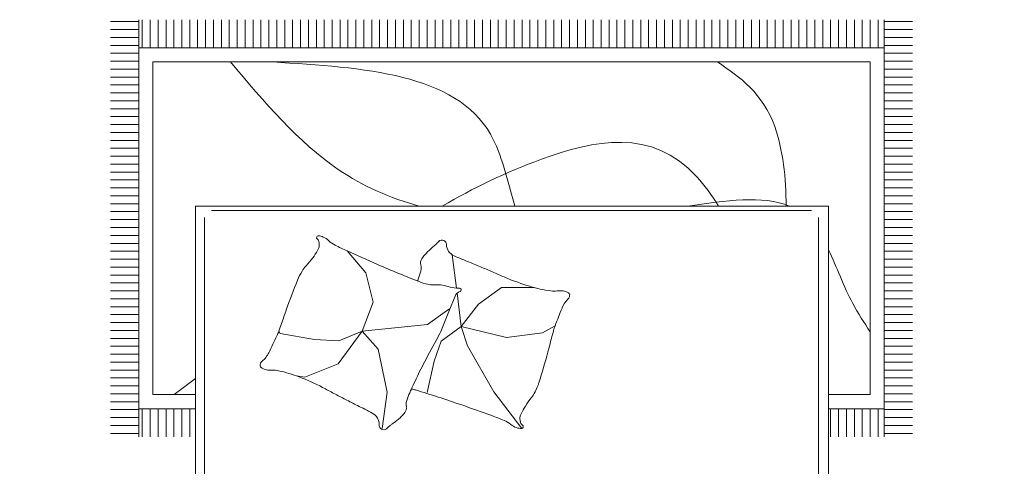
# Model space of a CAD drawing. Units: inches. Extents: x -7 to 1228, y -146 to 1091.
# Tile 46 of 88: x 81 to 168, y 616 to 655. Entities that reach past the tile are written whole.
import ezdxf

# ---------------------------------------------------------------- set-up
doc = ezdxf.new("R2010")
doc.units = ezdxf.units.IN
doc.layers.add('A-FURN', color=8, linetype='Continuous', lineweight=18)
doc.styles.add('DIM_FONT', font='SIMPLEX.shx', dxfattribs={"width": 0.8})

# ---------------------------------------------------------------- blocks, each defined once
blk = doc.blocks.new('A$C4F634EDD')
for p, q in [((0, 2.6295), (0, 2.2295)), ((0.5, 2.6295), (0, 2.6295)), ((0.5, 2.6295), (2.3, 2.6295)), ((0.5, 0.5295), (0.5, 2.6295)), ((0.5, 2.2295), (0.5, 2.6295)), ((2.3, 2.6295), (2.3, 0.5295)), ((2.3, 2.6295), (2.8, 2.6295)), ((2.3, 2.2295), (2.3, 2.6295)), ((2.8, 2.6295), (2.8, 2.2295)), ((0.5, 2.5771), (2.3, 2.5771)), ((2.392, 2.5115), (2.5692, 2.5765)), ((2.5692, 2.5765), (2.574, 2.5743)), ((0.2457, 2.5697), (0.2457, 2.4733)), ((2.4985, 2.5445), (2.5516, 2.564)), ((2.5062, 2.5454), (2.5487, 2.561)), ((2.5483, 2.5347), (2.5487, 2.561)), ((2.5487, 2.561), (2.5571, 2.56)), ((2.5615, 2.5536), (2.5514, 2.5318)), ((2.5516, 2.564), (2.5637, 2.5584)), ((2.5571, 2.56), (2.5615, 2.5536)), ((2.5615, 2.5536), (2.5791, 2.5058)), ((2.5637, 2.5584), (2.6418, 2.3458)), ((2.574, 2.5743), (2.6638, 2.3298)), ((2.4842, 2.5232), (2.47, 2.518)), ((2.4862, 2.5179), (2.4842, 2.5232)), ((2.4946, 2.5331), (2.4985, 2.5445)), ((2.5734, 2.3187), (2.4946, 2.5331)), ((2.5062, 2.5454), (2.5004, 2.5392)), ((2.5004, 2.5392), (2.5013, 2.5315)), ((2.5013, 2.5315), (2.5188, 2.4836)), ((2.5013, 2.5315), (2.5231, 2.5214)), ((2.5235, 2.5256), (2.5062, 2.5454)), ((2.5231, 2.5214), (2.5235, 2.5256)), ((2.5523, 2.4417), (2.5231, 2.5214)), ((2.5483, 2.5347), (2.5235, 2.5256)), ((2.5514, 2.5318), (2.5483, 2.5347)), ((2.5807, 2.4521), (2.5514, 2.5318)), ((2.3898, 2.5066), (2.392, 2.5115)), ((2.4795, 2.2621), (2.3898, 2.5066)), ((2.412, 2.5007), (2.4634, 2.5196)), ((2.4361, 2.4352), (2.412, 2.5007)), ((2.4634, 2.5196), (2.4875, 2.454)), ((2.47, 2.518), (2.472, 2.5127)), ((2.472, 2.5127), (2.4862, 2.5179)), ((2.4881, 2.5126), (2.4739, 2.5074)), ((2.4739, 2.5074), (2.4759, 2.502)), ((2.4759, 2.502), (2.4901, 2.5073)), ((2.492, 2.5019), (2.4778, 2.4967)), ((2.4778, 2.4967), (2.4798, 2.4914)), ((2.4798, 2.4914), (2.494, 2.4966)), ((2.4901, 2.5073), (2.4881, 2.5126)), ((2.494, 2.4966), (2.492, 2.5019)), ((2.5788, 2.4956), (2.5767, 2.4848)), ((2.5791, 2.5058), (2.5788, 2.4956)), ((2.4959, 2.4913), (2.4817, 2.4861)), ((2.4817, 2.4861), (2.4837, 2.4808)), ((2.4837, 2.4808), (2.4979, 2.486)), ((2.4998, 2.4807), (2.4856, 2.4755)), ((2.4856, 2.4755), (2.4876, 2.4702)), ((2.4876, 2.4702), (2.5018, 2.4754)), ((2.5037, 2.47), (2.4895, 2.4648)), ((2.4895, 2.4648), (2.4915, 2.4595)), ((2.4915, 2.4595), (2.5057, 2.4647)), ((2.4979, 2.486), (2.4959, 2.4913)), ((2.5018, 2.4754), (2.4998, 2.4807)), ((2.5057, 2.4647), (2.5037, 2.47)), ((2.5188, 2.4836), (2.5256, 2.4761)), ((2.5256, 2.4761), (2.5342, 2.4692)), ((2.5342, 2.4692), (2.5405, 2.4574)), ((2.5767, 2.4848), (2.5795, 2.4717)), ((2.5795, 2.4717), (2.586, 2.454)), ((2.4875, 2.454), (2.4361, 2.4352)), ((2.5405, 2.4574), (2.547, 2.4397)), ((2.5594, 2.4061), (2.547, 2.4397)), ((2.5523, 2.4417), (2.5875, 2.346)), ((2.5807, 2.4521), (2.6158, 2.3564)), ((2.5984, 2.4204), (2.586, 2.454)), ((0.0957, 2.4197), (0.192, 2.4197)), ((0.2994, 2.4197), (0.3957, 2.4197)), ((2.4457, 2.4146), (2.4563, 2.4185)), ((2.4496, 2.4039), (2.4457, 2.4146)), ((2.4563, 2.4185), (2.4602, 2.4078)), ((2.4634, 2.4211), (2.474, 2.425)), ((2.4673, 2.4104), (2.4634, 2.4211)), ((2.4779, 2.4143), (2.4673, 2.4104)), ((2.474, 2.425), (2.4779, 2.4143)), ((2.4811, 2.4276), (2.4917, 2.4315)), ((2.485, 2.4169), (2.4811, 2.4276)), ((2.4956, 2.4208), (2.485, 2.4169)), ((2.4883, 2.4081), (2.4989, 2.412)), ((2.4922, 2.3975), (2.4883, 2.4081)), ((2.4917, 2.4315), (2.4956, 2.4208)), ((2.4989, 2.412), (2.5028, 2.4014)), ((2.6047, 2.4086), (2.5984, 2.4204)), ((2.6133, 2.4017), (2.6047, 2.4086)), ((2.4602, 2.4078), (2.4496, 2.4039)), ((2.4528, 2.3951), (2.4635, 2.399)), ((2.4567, 2.3844), (2.4528, 2.3951)), ((2.4674, 2.3883), (2.4567, 2.3844)), ((2.4635, 2.399), (2.4674, 2.3883)), ((2.4706, 2.4016), (2.4812, 2.4055)), ((2.4745, 2.3909), (2.4706, 2.4016)), ((2.4851, 2.3949), (2.4745, 2.3909)), ((2.4777, 2.3821), (2.4883, 2.386)), ((2.4816, 2.3715), (2.4777, 2.3821)), ((2.4812, 2.4055), (2.4851, 2.3949)), ((2.4883, 2.386), (2.4922, 2.3754)), ((2.5028, 2.4014), (2.4922, 2.3975)), ((2.4954, 2.3886), (2.5061, 2.3925)), ((2.4993, 2.378), (2.4954, 2.3886)), ((2.51, 2.3819), (2.4993, 2.378)), ((2.5061, 2.3925), (2.51, 2.3819)), ((2.5238, 2.3769), (2.538, 2.3821)), ((2.538, 2.3821), (2.5419, 2.3715)), ((2.5622, 2.393), (2.5594, 2.4061)), ((2.5598, 2.372), (2.5601, 2.3822)), ((2.5601, 2.3822), (2.5622, 2.393)), ((2.6201, 2.3941), (2.6133, 2.4017)), ((2.6376, 2.3463), (2.6201, 2.3941)), ((2.6499, 2.3979), (2.6397, 2.3953)), ((2.6417, 2.39), (2.6488, 2.391)), ((2.6488, 2.391), (2.6538, 2.3895)), ((2.6551, 2.397), (2.6499, 2.3979)), ((2.6538, 2.3895), (2.6596, 2.388)), ((2.6627, 2.392), (2.6551, 2.397)), ((2.6596, 2.388), (2.6626, 2.3867)), ((2.6626, 2.3867), (2.6662, 2.388)), ((2.6692, 2.394), (2.6627, 2.392)), ((2.6662, 2.388), (2.6632, 2.3828)), ((2.6632, 2.3828), (2.6736, 2.3744)), ((2.6736, 2.3944), (2.6692, 2.394)), ((2.6765, 2.391), (2.6736, 2.3944)), ((2.6742, 2.3795), (2.6765, 2.391)), ((2.6824, 2.3858), (2.6742, 2.3795)), ((2.6873, 2.3815), (2.6824, 2.3858)), ((2.6853, 2.369), (2.6873, 2.3815)), ((0.2457, 2.366), (0.2457, 2.2697)), ((2.46, 2.3756), (2.4706, 2.3795)), ((2.4639, 2.365), (2.46, 2.3756)), ((2.4745, 2.3689), (2.4639, 2.365)), ((2.4672, 2.3561), (2.4778, 2.36)), ((2.4711, 2.3455), (2.4672, 2.3561)), ((2.4706, 2.3795), (2.4745, 2.3689)), ((2.4778, 2.36), (2.4817, 2.3494)), ((2.4922, 2.3754), (2.4816, 2.3715)), ((2.4849, 2.3626), (2.4955, 2.3665)), ((2.4888, 2.352), (2.4849, 2.3626)), ((2.4994, 2.3559), (2.4888, 2.352)), ((2.4955, 2.3665), (2.4994, 2.3559)), ((2.5026, 2.3691), (2.5132, 2.373)), ((2.5065, 2.3585), (2.5026, 2.3691)), ((2.5171, 2.3624), (2.5065, 2.3585)), ((2.5132, 2.373), (2.5171, 2.3624)), ((2.5277, 2.3663), (2.5238, 2.3769)), ((2.5419, 2.3715), (2.5277, 2.3663)), ((2.5774, 2.3242), (2.5598, 2.372)), ((2.6154, 2.3522), (2.5905, 2.3431)), ((2.6158, 2.3564), (2.6154, 2.3522)), ((2.6154, 2.3522), (2.6327, 2.3324)), ((2.6376, 2.3463), (2.6158, 2.3564)), ((2.6736, 2.3744), (2.6922, 2.3593)), ((2.6946, 2.376), (2.6853, 2.369)), ((2.6922, 2.3593), (2.7051, 2.3473)), ((2.6995, 2.3713), (2.6946, 2.376)), ((2.695, 2.3603), (2.6995, 2.3713)), ((2.7031, 2.3682), (2.695, 2.3603)), ((2.7096, 2.3616), (2.7031, 2.3682)), ((2.7062, 2.351), (2.7096, 2.3616)), ((2.7147, 2.3578), (2.7062, 2.351)), ((2.7214, 2.3517), (2.7147, 2.3578)), ((0, 2.3301), (0.5, 2.3301)), ((2.8, 2.3301), (2.3, 2.3301)), ((2.4817, 2.3494), (2.4711, 2.3455)), ((2.5774, 2.3242), (2.5875, 2.346)), ((2.5818, 2.3178), (2.5774, 2.3242)), ((2.5875, 2.346), (2.5905, 2.3431)), ((2.5905, 2.3431), (2.5901, 2.3168)), ((2.5901, 2.3168), (2.6097, 2.324)), ((2.613, 2.3312), (2.6077, 2.3293)), ((2.6077, 2.3293), (2.6135, 2.3141)), ((2.6192, 2.3174), (2.613, 2.3312)), ((2.6153, 2.3261), (2.6327, 2.3324)), ((2.6369, 2.332), (2.6161, 2.3243)), ((2.6616, 2.3249), (2.6234, 2.3109)), ((2.6327, 2.3324), (2.6385, 2.3386)), ((2.6418, 2.3458), (2.6369, 2.332)), ((2.6385, 2.3386), (2.6376, 2.3463)), ((2.6638, 2.3298), (2.6616, 2.3249)), ((2.7051, 2.3473), (2.7079, 2.3475)), ((2.7079, 2.3475), (2.7079, 2.3443)), ((2.7079, 2.3443), (2.727, 2.3277)), ((2.7196, 2.34), (2.7214, 2.3517)), ((2.7286, 2.3466), (2.7196, 2.34)), ((2.727, 2.3277), (2.7512, 2.2983)), ((2.7346, 2.3423), (2.7286, 2.3466)), ((2.732, 2.3295), (2.7346, 2.3423)), ((2.7423, 2.3345), (2.732, 2.3295)), ((2.7406, 2.3172), (2.7495, 2.325)), ((2.7495, 2.325), (2.7423, 2.3345)), ((2.6172, 2.3086), (2.4844, 2.2599)), ((2.5362, 2.305), (2.5185, 2.2985)), ((2.5185, 2.2985), (2.5224, 2.2879)), ((2.5401, 2.2944), (2.5362, 2.305)), ((2.561, 2.3141), (2.5433, 2.3076)), ((2.5433, 2.3076), (2.5472, 2.297)), ((2.5472, 2.297), (2.5649, 2.3035)), ((2.5649, 2.3035), (2.561, 2.3141)), ((2.5855, 2.3131), (2.5734, 2.3187)), ((2.5901, 2.3168), (2.5818, 2.3178)), ((2.6104, 2.3222), (2.5855, 2.3131)), ((2.6135, 2.3141), (2.6244, 2.2977)), ((2.626, 2.3069), (2.6192, 2.3174)), ((2.6244, 2.2977), (2.6349, 2.2825)), ((2.6365, 2.2916), (2.626, 2.3069)), ((2.7519, 2.3218), (2.7406, 2.3172)), ((2.7512, 2.2983), (2.756, 2.2695)), ((2.7575, 2.3144), (2.7519, 2.3218)), ((2.7526, 2.3045), (2.7575, 2.3144)), ((2.7622, 2.308), (2.7526, 2.3045)), ((2.7574, 2.2924), (2.7673, 2.2997)), ((2.7673, 2.2997), (2.7622, 2.308)), ((0.5953, 2.1912), (0.616, 2.2738)), ((1.4546, 2.1912), (1.4752, 2.2738)), ((2.5114, 2.2959), (2.4936, 2.2894)), ((2.4936, 2.2894), (2.4976, 2.2788)), ((2.4976, 2.2788), (2.5153, 2.2853)), ((2.5153, 2.2853), (2.5114, 2.2959)), ((2.5224, 2.2879), (2.5401, 2.2944)), ((2.6349, 2.2825), (2.638, 2.273)), ((2.6407, 2.2834), (2.6365, 2.2916)), ((2.6399, 2.2712), (2.6374, 2.2659)), ((2.638, 2.273), (2.6399, 2.2712)), ((2.6438, 2.2739), (2.6407, 2.2834)), ((2.6519, 2.2716), (2.6438, 2.2739)), ((2.6535, 2.2628), (2.6519, 2.2716)), ((2.756, 2.2695), (2.7459, 2.2483)), ((2.7687, 2.2905), (2.7574, 2.2924)), ((2.7587, 2.279), (2.7699, 2.2828)), ((2.7708, 2.2725), (2.7587, 2.279)), ((2.7699, 2.2828), (2.7687, 2.2905)), ((2.7706, 2.2643), (2.7708, 2.2725)), ((2.4844, 2.2599), (2.4795, 2.2621)), ((2.6374, 2.2659), (2.6398, 2.257)), ((2.6398, 2.257), (2.6509, 2.259)), ((2.6509, 2.259), (2.6431, 2.2492)), ((2.6431, 2.2492), (2.6473, 2.2398)), ((2.6473, 2.2398), (2.6592, 2.2429)), ((2.6592, 2.2429), (2.6521, 2.2314)), ((2.6636, 2.2409), (2.6535, 2.2628)), ((2.6836, 2.2287), (2.6636, 2.2409)), ((2.7459, 2.2483), (2.7284, 2.2317)), ((2.7509, 2.2314), (2.7459, 2.2418)), ((2.7459, 2.2418), (2.7568, 2.2352)), ((2.7529, 2.2505), (2.7645, 2.2498)), ((2.7607, 2.2424), (2.7529, 2.2505)), ((2.7568, 2.2352), (2.7607, 2.2424)), ((2.759, 2.2637), (2.7706, 2.2643)), ((2.7676, 2.2559), (2.759, 2.2637)), ((2.7645, 2.2498), (2.7676, 2.2559)), ((0, 2.2295), (0.5, 2.2295)), ((2.8, 2.2295), (2.3, 2.2295)), ((2.6521, 2.2314), (2.6598, 2.2248)), ((2.6598, 2.2248), (2.6697, 2.2309)), ((2.6697, 2.2309), (2.6684, 2.219)), ((2.6684, 2.219), (2.6761, 2.2145)), ((2.6761, 2.2145), (2.6821, 2.2237)), ((2.6821, 2.2237), (2.6843, 2.2135)), ((2.7063, 2.2256), (2.6836, 2.2287)), ((2.6843, 2.2135), (2.6927, 2.2117)), ((2.6927, 2.2117), (2.6986, 2.222)), ((2.6986, 2.222), (2.7019, 2.2098)), ((2.7284, 2.2317), (2.7063, 2.2256)), ((2.7102, 2.2104), (2.7113, 2.2218)), ((2.7113, 2.2218), (2.7192, 2.2137)), ((2.7192, 2.2137), (2.7255, 2.2152)), ((2.7255, 2.2152), (2.7242, 2.2265)), ((2.7242, 2.2265), (2.7324, 2.2165)), ((2.7324, 2.2165), (2.7386, 2.2208)), ((2.7386, 2.2208), (2.7354, 2.2306)), ((2.7354, 2.2306), (2.7462, 2.2264)), ((2.7462, 2.2264), (2.7509, 2.2314)), ((0.5878, 2.1612), (0.5953, 2.1912)), ((1.4471, 2.1612), (1.4546, 2.1912)), ((2.7019, 2.2098), (2.7102, 2.2104)), ((1.5035, 2.141), (0.5458, 2.141)), ((1.5035, 2.141), (2.2716, 1.7136)), ((0.5258, 2.121), (0.5258, 0.5617)), ((1.576, 1.9433), (1.5624, 1.8479)), ((0.5458, 1.8684), (1.5653, 1.8684)), ((1.5624, 1.8479), (1.5641, 1.7178)), ((2.2716, 0.5617), (2.2716, 1.7136)), ((0.3386, 0), (0.3386, 1.1852)), ((0.3486, 1.1052), (0.3486, 1.1852)), ((0.3711, 1.1052), (0.3711, 1.1852)), ((0.3936, 1.1052), (0.3936, 1.1852)), ((0.4161, 1.1052), (0.4161, 1.1852)), ((0.4386, 1.1052), (0.4386, 1.1852)), ((0.4611, 1.1052), (0.4611, 1.1852)), ((0.4836, 1.1052), (0.4836, 1.1852)), ((2.3061, 1.1052), (2.3061, 1.1852)), ((2.3286, 1.1052), (2.3286, 1.1852)), ((2.3511, 1.1052), (2.3511, 1.1852)), ((2.3736, 1.1052), (2.3736, 1.1852)), ((2.3961, 1.1052), (2.3961, 1.1852)), ((2.4186, 1.1052), (2.4186, 1.1852)), ((2.4411, 1.1052), (2.4411, 1.1852)), ((2.4588, 1.1852), (2.4588, 0)), ((0.2586, 1.1753), (0.3386, 1.1753)), ((0.2586, 1.1528), (0.3386, 1.1528)), ((1.031, 1.1612), (1.0448, 1.0581)), ((1.4276, 1.1611), (1.3484, 1.0571)), ((2.4588, 1.1753), (2.5388, 1.1753)), ((2.4588, 1.1528), (2.5388, 1.1528)), ((0.2586, 1.1303), (0.3386, 1.1303)), ((2.4588, 1.1303), (2.5388, 1.1303)), ((0.2586, 1.1078), (0.3386, 1.1078)), ((0.3386, 1.1052), (0.5, 1.1052)), ((2.3, 1.1052), (2.4588, 1.1052)), ((2.4588, 1.1078), (2.5388, 1.1078)), ((0.2586, 1.0853), (0.3386, 1.0853)), ((0.3786, 1.0652), (0.5, 1.0652)), ((0.3786, 0.12), (0.3786, 1.0652)), ((2.3, 1.0652), (2.4188, 1.0652)), ((2.4188, 1.0652), (2.4188, 0.12)), ((2.4588, 1.0853), (2.5388, 1.0853)), ((0.2586, 1.0628), (0.3386, 1.0628)), ((0.2586, 1.0403), (0.3386, 1.0403)), ((1.0448, 1.0581), (1.019, 0.936)), ((1.1784, 0.9702), (1.1586, 1.0591)), ((1.3484, 1.0571), (1.2733, 0.9268)), ((2.4588, 1.0628), (2.5388, 1.0628)), ((2.4588, 1.0403), (2.5388, 1.0403)), ((0.2586, 1.0178), (0.3386, 1.0178)), ((0.8108, 1.0151), (0.7868, 1.0117)), ((0.9054, 0.9773), (0.8108, 1.0151)), ((2.4588, 1.0178), (2.5388, 1.0178)), ((0.2586, 0.9953), (0.3386, 0.9953)), ((2.4588, 0.9953), (2.5388, 0.9953)), ((0.2586, 0.9728), (0.3386, 0.9728)), ((0.9743, 0.8845), (0.9054, 0.9773)), ((1.1982, 0.9129), (1.1784, 0.9702)), ((2.4588, 0.9728), (2.5388, 0.9728)), ((0.2586, 0.9503), (0.3386, 0.9503)), ((0.2586, 0.9278), (0.3386, 0.9278)), ((1.019, 0.936), (0.9743, 0.8845)), ((1.2733, 0.9268), (1.2555, 0.8715)), ((2.4588, 0.9503), (2.5388, 0.9503)), ((2.4588, 0.9278), (2.5388, 0.9278)), ((0.2586, 0.9053), (0.3386, 0.9053)), ((0.8384, 0.9085), (0.7403, 0.8913)), ((0.9072, 0.912), (0.8384, 0.9085)), ((0.9743, 0.8845), (0.9072, 0.912)), ((1.2555, 0.8715), (1.1982, 0.9129)), ((1.2555, 0.8715), (1.384, 0.9031)), ((1.384, 0.9031), (1.4868, 0.8892)), ((2.4588, 0.9053), (2.5388, 0.9053)), ((0.2586, 0.8828), (0.3386, 0.8828)), ((0.7403, 0.8913), (0.737, 0.8849)), ((0.9743, 0.8845), (1.0052, 0.802)), ((0.9743, 0.8845), (1.16, 0.8656)), ((1.1973, 0.8853), (1.2203, 0.829)), ((1.2555, 0.8715), (1.2437, 0.7773)), ((1.2555, 0.8715), (1.3049, 0.8082)), ((1.4868, 0.8892), (1.5228, 0.8692)), ((2.4588, 0.8828), (2.5388, 0.8828)), ((0.2586, 0.8603), (0.3386, 0.8603)), ((1.16, 0.8656), (1.2099, 0.8295)), ((2.4588, 0.8603), (2.5388, 0.8603)), ((0.2586, 0.8378), (0.3386, 0.8378)), ((0.2586, 0.8153), (0.3386, 0.8153)), ((1.2099, 0.8295), (1.222, 0.8209)), ((1.2203, 0.829), (1.2381, 0.7855)), ((2.4588, 0.8378), (2.5388, 0.8378)), ((2.4588, 0.8153), (2.5388, 0.8153)), ((0.2586, 0.7928), (0.3386, 0.7928)), ((1.0052, 0.802), (0.9846, 0.7194)), ((1.3049, 0.8082), (1.3701, 0.7608)), ((2.4588, 0.7928), (2.5388, 0.7928)), ((0.2586, 0.7703), (0.3386, 0.7703)), ((1.2419, 0.7626), (1.23, 0.668)), ((1.3701, 0.7608), (1.463, 0.7608)), ((2.4588, 0.7703), (2.5388, 0.7703)), ((0.2586, 0.7478), (0.3386, 0.7478)), ((2.4588, 0.7478), (2.5388, 0.7478)), ((0.2586, 0.7253), (0.3386, 0.7253)), ((0.2586, 0.7028), (0.3386, 0.7028)), ((0.9846, 0.7194), (0.931, 0.6569)), ((2.4588, 0.7253), (2.5388, 0.7253)), ((2.4588, 0.7028), (2.5388, 0.7028)), ((0.2586, 0.6803), (0.3386, 0.6803)), ((2.4588, 0.6803), (2.5388, 0.6803)), ((0.2586, 0.6578), (0.3386, 0.6578)), ((2.4588, 0.6578), (2.5388, 0.6578)), ((0.2586, 0.6353), (0.3386, 0.6353)), ((2.4588, 0.6353), (2.5388, 0.6353)), ((0.2586, 0.6128), (0.3386, 0.6128)), ((0.2586, 0.5903), (0.3386, 0.5903)), ((2.4588, 0.6128), (2.5388, 0.6128)), ((2.4588, 0.5903), (2.5388, 0.5903)), ((0.2586, 0.5678), (0.3386, 0.5678)), ((2.4588, 0.5678), (2.5388, 0.5678)), ((0.2586, 0.5453), (0.3386, 0.5453)), ((0.5458, 0.5417), (2.2516, 0.5417)), ((2.4588, 0.5453), (2.5388, 0.5453)), ((0.2586, 0.5228), (0.3386, 0.5228)), ((2.3, 0.5295), (0.5, 0.5295)), ((2.4588, 0.5228), (2.5388, 0.5228)), ((0.2586, 0.5003), (0.3386, 0.5003)), ((0.2586, 0.4778), (0.3386, 0.4778)), ((2.4588, 0.5003), (2.5388, 0.5003)), ((2.4588, 0.4778), (2.5388, 0.4778)), ((0.2586, 0.4553), (0.3386, 0.4553)), ((2.4588, 0.4553), (2.5388, 0.4553)), ((0.2586, 0.4328), (0.3386, 0.4328)), ((2.4588, 0.4328), (2.5388, 0.4328)), ((0.2586, 0.4103), (0.3386, 0.4103)), ((2.4588, 0.4103), (2.5388, 0.4103)), ((0.2586, 0.3878), (0.3386, 0.3878)), ((0.2586, 0.3653), (0.3386, 0.3653)), ((2.4588, 0.3878), (2.5388, 0.3878)), ((2.4588, 0.3653), (2.5388, 0.3653)), ((0.2586, 0.3428), (0.3386, 0.3428)), ((2.4588, 0.3428), (2.5388, 0.3428)), ((0.2586, 0.3203), (0.3386, 0.3203)), ((2.4588, 0.3203), (2.5388, 0.3203)), ((0.2586, 0.2978), (0.3386, 0.2978)), ((2.4588, 0.2978), (2.5388, 0.2978)), ((0.2586, 0.2753), (0.3386, 0.2753)), ((0.2586, 0.2528), (0.3386, 0.2528)), ((2.4588, 0.2753), (2.5388, 0.2753)), ((2.4588, 0.2528), (2.5388, 0.2528)), ((0.2586, 0.2303), (0.3386, 0.2303)), ((2.4588, 0.2303), (2.5388, 0.2303)), ((0.2586, 0.2078), (0.3386, 0.2078)), ((2.4588, 0.2078), (2.5388, 0.2078)), ((0.2586, 0.1853), (0.3386, 0.1853)), ((2.4588, 0.1853), (2.5388, 0.1853)), ((0.2586, 0.1628), (0.3386, 0.1628)), ((0.2586, 0.1403), (0.3386, 0.1403)), ((2.4588, 0.1628), (2.5388, 0.1628)), ((2.4588, 0.1403), (2.5388, 0.1403)), ((0.2586, 0.1178), (0.3386, 0.1178)), ((2.4188, 0.12), (0.3786, 0.12)), ((2.4588, 0.1178), (2.5388, 0.1178)), ((0.2586, 0.0953), (0.3386, 0.0953)), ((2.4588, 0.0953), (2.5388, 0.0953)), ((0.2586, 0.0728), (0.3386, 0.0728)), ((2.4588, 0.08), (0.3386, 0.08)), ((0.3486, 0), (0.3486, 0.08)), ((0.3711, 0), (0.3711, 0.08)), ((0.3936, 0), (0.3936, 0.08)), ((0.4161, 0), (0.4161, 0.08)), ((0.4386, 0), (0.4386, 0.08)), ((0.4611, 0), (0.4611, 0.08)), ((0.4836, 0), (0.4836, 0.08)), ((0.5061, 0), (0.5061, 0.08)), ((0.5286, 0), (0.5286, 0.08)), ((0.5511, 0), (0.5511, 0.08)), ((0.5736, 0), (0.5736, 0.08)), ((0.5961, 0), (0.5961, 0.08)), ((0.6186, 0), (0.6186, 0.08)), ((0.6411, 0), (0.6411, 0.08)), ((0.6636, 0), (0.6636, 0.08)), ((0.6861, 0), (0.6861, 0.08)), ((0.7086, 0), (0.7086, 0.08)), ((0.7311, 0), (0.7311, 0.08)), ((0.7536, 0), (0.7536, 0.08)), ((0.7761, 0), (0.7761, 0.08)), ((0.7986, 0), (0.7986, 0.08)), ((0.8211, 0), (0.8211, 0.08)), ((0.8436, 0), (0.8436, 0.08)), ((0.8661, 0), (0.8661, 0.08)), ((0.8886, 0), (0.8886, 0.08)), ((0.9111, 0), (0.9111, 0.08)), ((0.9336, 0), (0.9336, 0.08)), ((0.9561, 0), (0.9561, 0.08)), ((0.9786, 0), (0.9786, 0.08)), ((1.0011, 0), (1.0011, 0.08)), ((1.0236, 0), (1.0236, 0.08)), ((1.0461, 0), (1.0461, 0.08)), ((1.0686, 0), (1.0686, 0.08)), ((1.0911, 0), (1.0911, 0.08)), ((1.1136, 0), (1.1136, 0.08)), ((1.1361, 0), (1.1361, 0.08)), ((1.1586, 0), (1.1586, 0.08)), ((1.1811, 0), (1.1811, 0.08)), ((1.2036, 0), (1.2036, 0.08)), ((1.2261, 0), (1.2261, 0.08)), ((1.2486, 0), (1.2486, 0.08)), ((1.2711, 0), (1.2711, 0.08)), ((1.2936, 0), (1.2936, 0.08)), ((1.3161, 0), (1.3161, 0.08)), ((1.3386, 0), (1.3386, 0.08)), ((1.3611, 0), (1.3611, 0.08)), ((1.3836, 0), (1.3836, 0.08)), ((1.4061, 0), (1.4061, 0.08)), ((1.4286, 0), (1.4286, 0.08)), ((1.4511, 0), (1.4511, 0.08)), ((1.4736, 0), (1.4736, 0.08)), ((1.4961, 0), (1.4961, 0.08)), ((1.5186, 0), (1.5186, 0.08)), ((1.5411, 0), (1.5411, 0.08)), ((1.5636, 0), (1.5636, 0.08)), ((1.5861, 0), (1.5861, 0.08)), ((1.6086, 0), (1.6086, 0.08)), ((1.6311, 0), (1.6311, 0.08)), ((1.6536, 0), (1.6536, 0.08)), ((1.6761, 0), (1.6761, 0.08)), ((1.6986, 0), (1.6986, 0.08)), ((1.7211, 0), (1.7211, 0.08)), ((1.7436, 0), (1.7436, 0.08)), ((1.7661, 0), (1.7661, 0.08)), ((1.7886, 0), (1.7886, 0.08)), ((1.8111, 0), (1.8111, 0.08)), ((1.8336, 0), (1.8336, 0.08)), ((1.8561, 0), (1.8561, 0.08)), ((1.8786, 0), (1.8786, 0.08)), ((1.9011, 0), (1.9011, 0.08)), ((1.9236, 0), (1.9236, 0.08)), ((1.9461, 0), (1.9461, 0.08)), ((1.9686, 0), (1.9686, 0.08)), ((1.9911, 0), (1.9911, 0.08)), ((2.0136, 0), (2.0136, 0.08)), ((2.0361, 0), (2.0361, 0.08)), ((2.0586, 0), (2.0586, 0.08)), ((2.0811, 0), (2.0811, 0.08)), ((2.1036, 0), (2.1036, 0.08)), ((2.1261, 0), (2.1261, 0.08)), ((2.1486, 0), (2.1486, 0.08)), ((2.1711, 0), (2.1711, 0.08)), ((2.1936, 0), (2.1936, 0.08)), ((2.2161, 0), (2.2161, 0.08)), ((2.2386, 0), (2.2386, 0.08)), ((2.2611, 0), (2.2611, 0.08)), ((2.2836, 0), (2.2836, 0.08)), ((2.3061, 0), (2.3061, 0.08)), ((2.3286, 0), (2.3286, 0.08)), ((2.3511, 0), (2.3511, 0.08)), ((2.3736, 0), (2.3736, 0.08)), ((2.3961, 0), (2.3961, 0.08)), ((2.4186, 0), (2.4186, 0.08)), ((2.4411, 0), (2.4411, 0.08)), ((2.4588, 0.0728), (2.5388, 0.0728)), ((0.2586, 0.0503), (0.3386, 0.0503)), ((2.4588, 0.0503), (2.5388, 0.0503)), ((0.2586, 0.0278), (0.3386, 0.0278)), ((0.2586, 0.0053), (0.3386, 0.0053)), ((2.4588, 0.0278), (2.5388, 0.0278)), ((2.4588, 0.0053), (2.5388, 0.0053))]:
    blk.add_line(p, q)
for radius in [0.1222, 0.0865]:
    blk.add_circle((0.2457, 2.4197), radius)
for centre, radius, start, end in [((0.5848, 2.5274), 0.0131, 101.2724, 206.5805), ((0.6036, 2.5368), 0.0342, 206.5805, 265.5998), ((0.5999, 2.4516), 0.0904, 90, 101.2724), ((0.5999, 2.3808), 0.1611, 81.5628, 90), ((0.5788, 2.2388), 0.3048, 74.256, 81.5628), ((0.7272, 2.7653), 0.2422, 254.256, 262.4531), ((0.7851, 3.2019), 0.6827, 262.4531, 270), ((0.7851, 3.5682), 1.049, 270, 276.0867), ((0.8402, 3.0514), 0.5293, 276.0867, 280.1899), ((1.1602, -8.1346), 10.6675, 90.30153, 91.21582), ((1.1169, 2.2433), 0.2897, 85.1982, 92.5386), ((1.2142, 3.4021), 0.8732, 265.1982, 269.4243), ((1.3082, 2.3102), 0.234, 110.8603, 117.2396), ((1.2204, 4.0232), 1.4943, 269.4243, 271.9079), ((1.2995, 2.4357), 0.0992, 105.9352, 126.0864), ((1.2429, 3.3501), 0.8208, 271.9079, 275.2592), ((1.2995, 2.4357), 0.0992, 85.7841, 105.9352), ((1.3132, 2.5864), 0.0539, 275.2592, 300.6513), ((1.3554, 2.5152), 0.0289, 85.6975, 120.6513), ((1.3556, 2.519), 0.0251, 68.2117, 85.6975), ((1.3739, 2.5288), 0.0156, 158.0096, 201.421), ((1.3634, 2.533), 0.00428, 78.1069, 158.0096), ((1.3288, 2.5111), 0.0328, 351.8665, 21.421), ((1.3647, 2.5395), 0.00232, 258.1069, 19.564), ((1.3637, 2.5391), 0.00342, 19.564, 68.2117), ((1.444, 2.5274), 0.0131, 101.2724, 206.5805), ((1.4628, 2.5368), 0.0342, 206.5805, 265.5998), ((1.4591, 2.4516), 0.0904, 90, 101.2724), ((1.4591, 2.3808), 0.1611, 81.5628, 90), ((1.438, 2.2388), 0.3048, 74.256, 81.5628), ((1.5865, 2.7653), 0.2422, 254.256, 262.4531), ((1.6443, 3.2019), 0.6827, 262.4531, 270), ((1.6443, 3.5682), 1.049, 270, 276.0867), ((1.4785, 15.4878), 12.9656, 271.22425, 272.05324), ((1.97, 2.3805), 0.1524, 92.5386, 100.1899), ((1.9761, 2.2433), 0.2897, 85.1982, 92.5386), ((2.0734, 3.4021), 0.8732, 265.1982, 269.4243), ((2.1674, 2.3102), 0.234, 110.8603, 117.2396), ((2.0797, 4.0232), 1.4943, 269.4243, 271.9079), ((2.1588, 2.4357), 0.0992, 105.9352, 126.0864), ((2.1021, 3.3501), 0.8208, 271.9079, 275.2592), ((2.1588, 2.4357), 0.0992, 85.7841, 105.9352), ((2.1724, 2.5864), 0.0539, 275.2592, 300.6513), ((2.2146, 2.5152), 0.0289, 85.6975, 120.6513), ((2.2149, 2.519), 0.0251, 68.2117, 85.6975), ((2.2331, 2.5288), 0.0156, 158.0096, 201.421), ((2.2226, 2.533), 0.00428, 78.1069, 158.0096), ((2.1881, 2.5111), 0.0328, 351.8665, 21.421), ((2.224, 2.5395), 0.00232, 258.1069, 19.564), ((2.2229, 2.5391), 0.00342, 19.564, 68.2117), ((1.0898, 2.4496), 0.4918, 173.7676, 180), ((0.5368, 2.3783), 0.1399, 45.0976, 62.7964), ((1.4317, 2.2032), 0.3916, 128.3886, 133.8115), ((1.2362, 2.45), 0.0768, 117.2396, 128.3886), ((1.2995, 2.4357), 0.0992, 143.8234, 161.5603), ((1.2995, 2.4357), 0.0992, 126.0864, 143.8234), ((1.1177, 2.5413), 0.246, 347.8905, 351.8665), ((1.949, 2.4496), 0.4918, 173.7676, 180), ((2.291, 2.2032), 0.3916, 128.3886, 133.8115), ((2.0954, 2.45), 0.0768, 117.2396, 128.3886), ((2.1588, 2.4357), 0.0992, 143.8234, 161.5603), ((2.1588, 2.4357), 0.0992, 126.0864, 143.8234), ((1.977, 2.5413), 0.246, 347.8905, 351.8665), ((0.5462, 2.4142), 0.0899, 41.4429, 53.7359), ((0.5741, 2.4389), 0.0526, 25.3551, 41.4429), ((0.5368, 2.3783), 0.1399, 27.3988, 45.0976), ((1.1799, 2.4341), 0.0493, 140.9651, 151.6832), ((1.3165, 2.3233), 0.2252, 133.8115, 140.9651), ((2.2605, 2.3525), 0.9131, 172.3191, 176.6313), ((1.5522, 2.448), 0.1983, 167.8905, 172.3191), ((2.0391, 2.4341), 0.0493, 140.9651, 151.6832), ((2.1757, 2.3233), 0.2252, 133.8115, 140.9651), ((3.1198, 2.3525), 0.9131, 172.3191, 176.6313), ((2.4114, 2.448), 0.1983, 167.8905, 172.3191), ((0.8019, 2.4496), 0.204, 180, 189.6844), ((0.4851, 2.3967), 0.1511, 21.8149, 25.3551), ((0.4345, 2.3765), 0.2056, 18.7799, 21.8149), ((0.576, 2.4246), 0.0562, 0, 18.7799), ((0.5368, 2.3783), 0.1399, 16.515, 27.3988), ((1.3127, 2.3625), 0.2002, 151.6832, 156.9972), ((1.6611, 2.4496), 0.204, 180, 189.6844), ((2.1719, 2.3625), 0.2002, 151.6832, 156.9972), ((1.4703, 2.5637), 0.882, 189.6844, 192.1984), ((0.5406, 2.4246), 0.0915, 345.3149, 0), ((0.5368, 2.3783), 0.1399, 5.6311, 16.515), ((2.3295, 2.5637), 0.882, 189.6844, 192.1984), ((2.0266, 2.3663), 0.6787, 176.6313, 181.6331), ((2.8858, 2.3663), 0.6787, 176.6313, 181.6331), ((0.2982, 2.3103), 0.3171, 8.0051, 12.1984), ((-0.0401, 2.2627), 0.6588, 2.6649, 8.0051), ((1.1575, 2.3103), 0.3171, 8.0051, 12.1984), ((0.8191, 2.2627), 0.6588, 2.6649, 8.0051), ((2.7128, 2.3859), 1.3652, 181.6331, 183.055), ((3.5721, 2.3859), 1.3652, 181.6331, 183.055), ((14.9657, 3.0398), 13.6356, 183.05496, 183.50486), ((15.8249, 3.0398), 13.6356, 183.05496, 183.50486), ((0.5503, 2.2902), 0.0677, 345.9548, 2.6649), ((1.4096, 2.2902), 0.0677, 345.9548, 2.6649), ((1.1303, 1.9835), 0.2721, 85.9172, 93.5552), ((1.1455, 2.197), 0.058, 69.3257, 85.9172), ((0.9871, 1.7772), 0.5066, 65.6735, 69.3257), ((0.473, 2.8815), 0.7387, 293.4844, 295.3111), ((0.6058, 0.9338), 1.4323, 63.5015, 65.6735), ((1.1054, 1.9358), 0.3126, 57.865, 63.5015), ((1.3322, 2.8815), 0.7387, 293.4844, 295.3111), ((0.473, 2.8815), 0.7387, 287.1982, 289.428), ((0.473, 2.8815), 0.7387, 289.428, 291.6577), ((0.473, 2.8815), 0.7387, 291.6577, 293.4844), ((0.8841, 1.5835), 0.7286, 54.1737, 57.865), ((1.6762, 2.2258), 0.3212, 183.5049, 189.9984), ((1.3322, 2.8815), 0.7387, 287.1982, 289.428), ((1.3322, 2.8815), 0.7387, 289.428, 291.6577), ((1.3322, 2.8815), 0.7387, 291.6577, 293.4844), ((2.5355, 2.2258), 0.3212, 183.5049, 189.9984), ((0.5887, 2.1609), 0.000917, 165.9551, 274.0829), ((0.5695, 2.4301), 0.2708, 274.0829, 279.4841), ((0.5763, 2.3896), 0.2297, 279.4841, 287.3864), ((0.6807, 2.0561), 0.1197, 96.4341, 107.3864), ((0.6836, 2.0301), 0.1459, 78.4414, 96.4341), ((0.759, 2.3985), 0.2301, 258.4414, 272.7491), ((0.7026, 3.5718), 1.4048, 272.7491, 274.6176), ((0.9136, 0.9591), 1.2165, 92.6096, 94.6176), ((1.2501, -19.8405), 22.0183, 90.37908, 91.01965), ((1.2012, -3.5404), 5.7185, 89.7135, 90.9704), ((1.224, 1.0141), 1.164, 86.426, 89.7135), ((1.2875, 2.0302), 0.1459, 77.131, 86.426), ((1.3099, 2.1283), 0.0453, 62.7159, 77.131), ((1.3658, 2.2367), 0.0767, 242.7159, 253.7788), ((1.3688, 2.247), 0.0875, 253.7788, 262.8796), ((1.3581, 2.1615), 0.00132, 262.8796, 343.3022), ((1.3409, 2.1667), 0.0193, 343.3022, 9.9984), ((1.448, 2.1609), 0.000917, 165.9551, 274.0829), ((1.4288, 2.4301), 0.2708, 274.0829, 279.4841), ((1.4355, 2.3896), 0.2297, 279.4841, 287.3864), ((1.5399, 2.0561), 0.1197, 96.4341, 107.3864), ((1.5429, 2.0301), 0.1459, 78.4414, 96.4341), ((1.6182, 2.3985), 0.2301, 258.4414, 272.7491), ((1.5619, 3.5718), 1.4048, 272.7491, 274.6176), ((1.7729, 0.9591), 1.2165, 92.6096, 94.6176), ((2.1093, -19.8405), 22.0183, 90.37908, 91.01965), ((2.0605, -3.5404), 5.7185, 89.7135, 90.9704), ((2.0833, 1.0141), 1.164, 86.426, 89.7135), ((2.1467, 2.0302), 0.1459, 77.131, 86.426), ((2.1691, 2.1283), 0.0453, 62.7159, 77.131), ((2.2251, 2.2367), 0.0767, 242.7159, 253.7788), ((2.2281, 2.247), 0.0875, 253.7788, 262.8796), ((2.2174, 2.1615), 0.00132, 262.8796, 343.3022), ((2.2001, 2.1667), 0.0193, 343.3022, 9.9984), ((0.5458, 2.121), 0.02, 90, 180), ((1.2147, 1.9017), 0.3751, 20.1488, 39.6445), ((1.3977, 1.9688), 0.1801, 351.8644, 20.1488), ((0.5458, 1.8884), 0.02, 180, 270), ((1.4194, 4.2174), 2.5158, 281.6741, 283.1904), ((2.0378, 1.5789), 0.1942, 97.7304, 103.1904), ((2.0195, 1.7137), 0.0581, 79.2724, 97.7304), ((1.2737, -2.2227), 4.0646, 77.0745, 79.2724), ((0.6102, 18.0525), 16.3521, 273.75703, 274.62393), ((2.0359, 1.0981), 0.6574, 74.0648, 77.0745), ((1.0582, 5.4638), 3.7801, 277.692, 279.495), ((1.7125, -0.0344), 1.8351, 72.2636, 74.0648), ((0.9863, 1.1494), 0.0359, 297.2902, 3.2455), ((1.0348, 1.1521), 0.0127, 51.1864, 183.2455), ((0.9991, 1.1077), 0.0697, 45.8726, 51.1864), ((1.0791, 1.1902), 0.0452, 225.8726, 232.4713), ((1.2846, 1.4577), 0.3825, 232.4713, 233.7837), ((0.6683, 0.6162), 0.6605, 52.7849, 53.7837), ((1.3469, 1.2115), 0.0792, 292.7069, 308.5854), ((1.4338, 1.1026), 0.0601, 110.3452, 128.5854), ((1.4251, 1.1259), 0.0352, 86.0516, 110.3452), ((1.4376, 1.1398), 0.0142, 126.5792, 169.5926), ((1.4273, 1.1567), 0.00443, 13.2808, 86.0516), ((1.4254, 1.1562), 0.0063, 306.5792, 13.2808), ((0.9362, 0.9689), 0.2176, 46.4776, 52.7849), ((1.0327, 1.0706), 0.0774, 35.8936, 46.4776), ((-0.4107, 5.9078), 5.0942, 289.0836, 290.1287), ((1.0543, 1.9106), 0.8371, 290.1287, 292.7069), ((1.4996, 1.1284), 0.0771, 169.5926, 177.2714), ((1.4378, 1.1314), 0.0153, 177.2714, 194.5709), ((1.4611, 1.1374), 0.0393, 194.5709, 206.8179), ((1.8575, -0.7096), 2.0162, 116.4147, 117.4999), ((-0.4173, 3.8699), 3.0972, 296.4147, 297.2902), ((1.0771, 1.1027), 0.0226, 351.9508, 35.8936), ((1.1449, 1.0931), 0.0458, 171.9508, 202.4162), ((0.2266, 4.0657), 3.145, 286.6085, 289.0836), ((1.7401, 1.2785), 0.352, 206.8179, 210.9056), ((1.6045, 1.1973), 0.194, 210.9056, 219.7005), ((3.744, -4.3336), 6.1019, 117.49986, 117.84822), ((2.032, 1.4591), 1.0054, 202.4162, 205.0529), ((1.3929, 1.0217), 0.081, 26.0735, 39.7005), ((0.5736, 1.5979), 0.6236, 290.7486, 297.4921), ((-1.8336, 6.2238), 5.8383, 297.49208, 297.84822), ((1.0922, 1.1636), 0.1166, 280.7366, 286.6085), ((1.2892, 0.9709), 0.1965, 17.8396, 26.0735), ((0.6422, 1.4168), 0.43, 282.6252, 290.7486), ((2.6493, 1.7476), 1.6868, 205.0529, 207.0884), ((-0.4304, 0.4175), 2.003, 15.2625, 17.8396), ((0.6894, 0.9832), 0.0058, 121.6917, 179.0386), ((0.7004, 0.983), 0.0168, 179.0386, 229.4914), ((0.7131, 0.9448), 0.0509, 103.0402, 121.6917), ((0.7152, 0.9361), 0.0599, 86.6119, 103.0402), ((0.7224, 1.0587), 0.063, 266.6119, 282.6252), ((0.6405, 0.9128), 0.0755, 26.3332, 49.4914), ((2.541, 1.6922), 1.5652, 207.0884, 209.936), ((-1.6775, -0.2344), 2.6619, 25.1732, 26.3332), ((-0.0881, 0.5109), 1.6481, 13.841, 15.2625), ((0.5689, 0.8213), 0.1798, 20.7081, 25.1732), ((0.9989, 0.8042), 0.2143, 22.2355, 29.936), ((2.0418, 1.0357), 0.5454, 193.841, 196.3122), ((0.2268, 0.692), 0.5454, 18.2369, 20.7081), ((1.6908, 0.933), 0.1798, 196.3122, 200.7773), ((4.0115, 1.8135), 2.6619, 200.7773, 201.9373), ((2.3102, 1.3785), 1.6481, 198.2369, 199.6584), ((2.6444, 1.4979), 2.003, 199.6584, 202.2355), ((1.6124, 0.8472), 0.0755, 201.9373, 225.0955), ((1.2594, 0.7942), 0.0231, 202.2355, 252.8133), ((1.5473, 0.7819), 0.0168, 354.6428, 45.0955), ((1.1727, 0.9313), 0.1794, 277.6784, 284.8807), ((1.2689, 0.569), 0.1955, 97.9822, 104.8807), ((1.2465, 0.729), 0.034, 85.7407, 97.9822), ((1.2497, 0.772), 0.0092, 265.7407, 289.3799), ((1.2512, 0.7678), 0.00467, 289.3799, 72.8133), ((1.6266, 0.159), 0.6236, 106.3527, 113.0962), ((1.5721, 0.3449), 0.43, 98.2293, 106.3527), ((1.5195, 0.708), 0.063, 82.216, 98.2293), ((1.5362, 0.8298), 0.0599, 262.216, 278.6443), ((1.5375, 0.8209), 0.0509, 278.6443, 297.2959), ((1.5582, 0.7808), 0.0058, 297.2959, 354.6428), ((0.9722, 0.8143), 0.1965, 202.2355, 210.4694), ((2.2689, -2.1899), 3.145, 111.0043, 113.4795), ((0.1831, 0.4093), 1.0054, 18.0203, 19.3448), ((1.1834, 0.6373), 0.1166, 98.1216, 111.0043), ((1.1763, 0.687), 0.0663, 85.4882, 98.1216), ((1.1871, 0.8241), 0.0712, 265.4882, 277.6784), ((3.6722, -4.6377), 5.8383, 113.0962, 113.45234), ((0.8727, 0.7557), 0.081, 210.4694, 224.0964), ((1.0957, 0.7061), 0.0458, 347.5549, 18.0203), ((0.5234, 2.5582), 2.0162, 292.0188, 293.104), ((-1.0798, 6.3161), 6.1019, 293.10398, 293.45234), ((0.6752, 0.5644), 0.194, 35.3015, 44.0964), ((0.5462, 0.4731), 0.352, 31.2138, 35.3015), ((3.0455, -3.9778), 5.0942, 113.4795, 114.5246), ((1.1625, 0.6914), 0.0226, 167.5549, 211.4977), ((1.2092, 0.72), 0.0774, 211.4977, 222.0817), ((2.4404, -2.1823), 3.0972, 112.0188, 112.8944), ((0.8136, 0.6351), 0.0393, 18.9668, 31.2138), ((0.8364, 0.6429), 0.0153, 1.6673, 18.9668), ((1.2784, -0.1047), 0.8371, 114.5246, 117.1028), ((1.3133, 0.814), 0.2176, 222.0817, 228.389), ((1.6074, 1.1451), 0.6605, 228.389, 229.3878), ((1.2495, 0.6379), 0.0359, 112.8944, 178.8496), ((0.8506, 0.6191), 0.0063, 130.9751, 197.6767), ((0.8488, 0.6185), 0.00443, 197.6767, 270.4475), ((0.8372, 0.6345), 0.0142, 310.9751, 353.9885), ((0.8486, 0.6493), 0.0352, 270.4475, 294.7411), ((0.7746, 0.6411), 0.0771, 353.9885, 1.6673), ((0.8382, 0.6719), 0.0601, 294.7411, 312.9813), ((0.9332, 0.57), 0.0792, 117.1028, 132.9813), ((0.9284, 0.3533), 0.3825, 48.0754, 49.3878), ((1.1538, 0.6043), 0.0452, 41.4767, 48.0754), ((1.2399, 0.6804), 0.0697, 221.4767, 226.7905), ((1.2009, 0.6389), 0.0127, 226.7905, 358.8496)]:
    blk.add_arc(centre, radius, start, end)
for points in [[(0.4393, 1.0652), (0.4595, 1.05), (0.4798, 1.0348), (0.5, 1.0195)], [(1.9003, 0.5295), (2.0065, 0.514), (2.1132, 0.4978), (2.1894, 0.5295)]]:
    blk.add_open_spline(points, degree=3)
for points, knots in [([(2.3, 0.6535), (2.3236, 0.7026), (2.3554, 0.7914), (2.4015, 0.8608), (2.4188, 0.8868)], [1893.525221, 1893.525221, 1893.525221, 1893.525221, 2051.902476, 2146.74457, 2146.74457, 2146.74457, 2146.74457]), ([(0.5992, 0.12), (0.6957, 0.2341), (0.8523, 0.4189), (1.0536, 0.5069), (1.136, 0.5295)], [0, 0, 0, 0, 432.822832, 701.445452, 701.445452, 701.445452, 701.445452]), ([(0.7187, 0.12), (0.9791, 0.1362), (1.326, 0.1577), (1.3868, 0.4574), (1.408, 0.5295)], [0, 0, 0, 0, 653.160442, 870.050857, 870.050857, 870.050857, 870.050857]), ([(1.2016, 0.5295), (1.2892, 0.479), (1.5144, 0.3684), (1.8265, 0.2994), (1.9681, 0.4992), (1.9875, 0.5295)], [936.534237, 936.534237, 936.534237, 936.534237, 1243.285375, 1683.261222, 1758.254386, 1758.254386, 1758.254386, 1758.254386]), ([(2.1796, 0.5295), (2.1798, 0.4519), (2.1548, 0.2369), (2.0487, 0.164), (1.9846, 0.12)], [2202.034493, 2202.034493, 2202.034493, 2202.034493, 2357.807635, 2594.446174, 2594.446174, 2594.446174, 2594.446174])]:
    blk.add_open_spline(points, degree=3, knots=knots)
at = {"style": 'DIM_FONT', "width": 0.8, "flags": 9}
for tag, p in [('YSIZE', (0.5, 2.6295)), ('XSIZE', (0.5, 2.6295)), ('XSIZE', (2.2985, 2.6295)), ('YSIZE', (2.2985, 2.6295))]:
    blk.add_attdef(tag, p, '', height=0.0005, dxfattribs=at)

msp = doc.modelspace()

# ---------------------------------------------------------------- block references
at = {"layer": 'A-FURN', "xscale": -30.79356024027943, "yscale": 30.79356024027943, "zscale": 30.79356024027943, "rotation": 180}
msp.add_blockref('A$C4F634EDD', (81.405, 654.972), dxfattribs=at)

doc.saveas('drawing.dxf')
